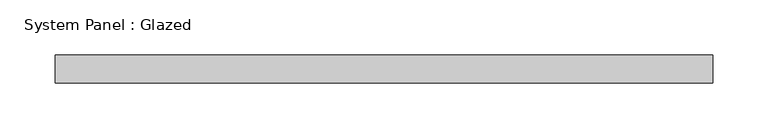
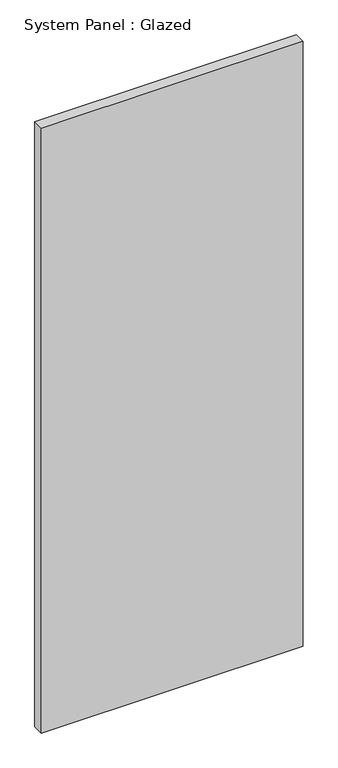
"""IFC4 building model written with IfcOpenShell, lengths in millimetres: plate geometry, System Panel : Glazed."""

from ifc_helpers import new_model, si_unit, origin, origin_with_axes, place, context, project, spatial, polyline, outline, extrude, source, transform, mapped, element, save


def system_panel_glazed_c0907c48(model_context):
    return source(origin(), model_context, "Body", "SweptSolid", [
        extrude(outline(polyline([(298.45, 19.05), (-298.45, 19.05), (-298.45, 44.45), (298.45, 44.45), (298.45, 19.05)])), origin_with_axes(), (0.0, 0.0, 1.0), 1457.3599864),
    ])


if __name__ == "__main__":
    model = new_model("IFC4")
    model_context = context("Model", 3, world=origin())
    ifc_project = project(units=[si_unit("LENGTHUNIT", "METRE", prefix="MILLI")], contexts=[model_context])
    site = spatial("IfcSite", under=ifc_project)
    building = spatial("IfcBuilding", under=site)
    placement = place(None, origin())
    system_panel_glazed_shape = system_panel_glazed_c0907c48(model_context)
    element("IfcPlate", 1, ObjectType="System Panel : Glazed", at=placement, inside=building, context=model_context, shape_type="MappedRepresentation", body=[
        mapped(system_panel_glazed_shape, transform((0.0, 0.0, 0.0), x_axis=(1.0, 0.0, 0.0), y_axis=(0.0, 1.0, 0.0), z_axis=(0.0, 0.0, 1.0))),
    ])
    save(model, "model.ifc")

# Revit data of these elements
# Type "System Panel : Glazed"
#   Construction Type Id = "GSP4R"
#   Analytic Construction = "1/8 in Pilkington single glazing"
#   Visual Light Transmittance = 0.9
#   Solar Heat Gain Coefficient = 0.86
#   Heat Transfer Coefficient (U) = 1.18115 BTU/(h·ft²·°F)
#   Define Thermal Properties by = 1
# Element 1 (IfcPlate, "System Panel : Glazed")
#   Materials on its faces: "Glass"
# Materials
#   "Glass": class "Glass", colour RGB 0 128 192, transparency 0.75, Description = "Soda Lime Glass", Cost = 0
